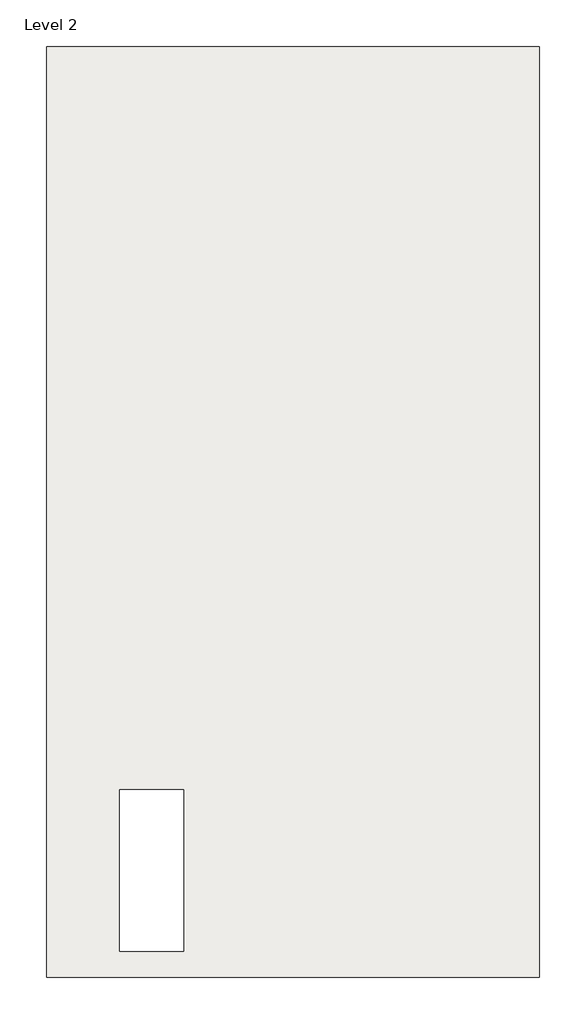
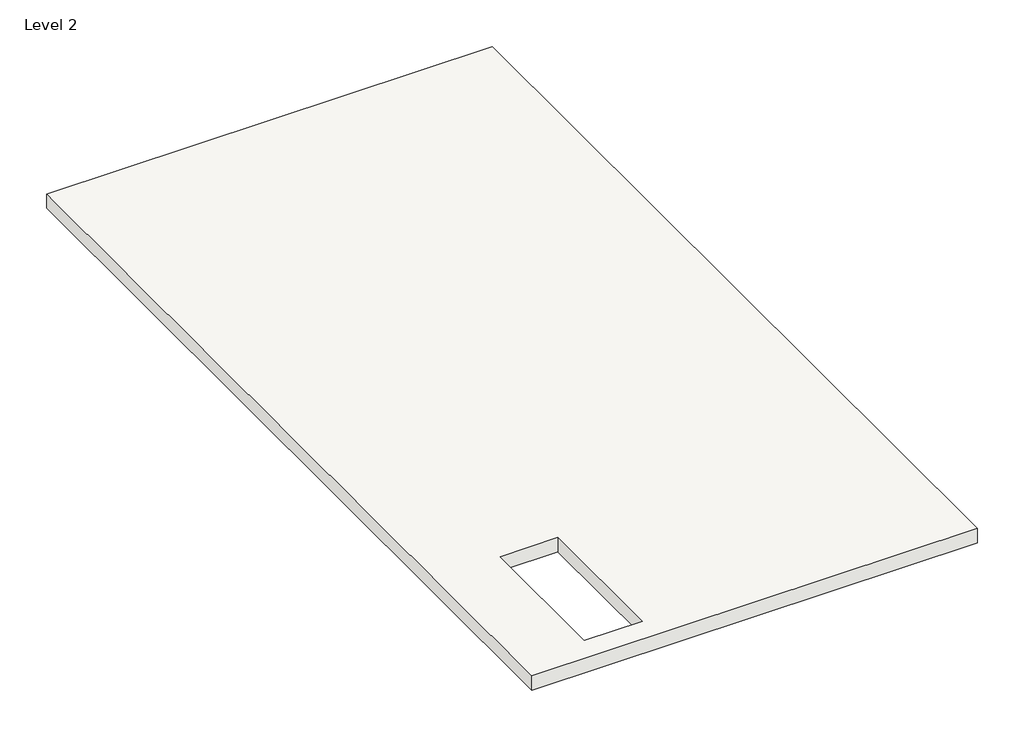
# One storey: 1 roof.
"""IFC4 building model written with IfcOpenShell, lengths in millimetres."""

from ifc_helpers import new_model, si_unit, frame, origin, place, context, project, spatial, polyline, outline, extrude, element, save

model = new_model("IFC4")

# Units and contexts
model_context = context("Model", 3, world=origin())
ifc_project = project(units=[si_unit("LENGTHUNIT", "METRE", prefix="MILLI")], contexts=[model_context])

# Site, building, storey
site = spatial("IfcSite", under=ifc_project)
building = spatial("IfcBuilding", under=site)
storey = spatial("IfcBuildingStorey", under=building, Name="Level 2", Elevation=3048.0)

# Roof
placement = place(None, origin())
element("IfcRoof", 1, ObjectType="Generic - 12\"", at=placement, inside=storey, context=model_context, shape_type="SweptSolid", body=[
    extrude(outline(polyline([(-13227.6589543, 12303.047818), (-4236.0589543, 12303.047818), (-4236.0589543, -4664.152182), (-13227.6589543, -4664.152182), (-13227.6589543, 12303.047818)]), holes=[polyline([(-11894.1589543, -1238.8838739), (-11894.1589543, -4185.2838739), (-10725.7589543, -4185.2838739), (-10725.7589543, -1238.8838739), (-11894.1589543, -1238.8838739)])]), frame((0.0, 0.0, 3048.0), z_axis=(0.0, 0.0, 1.0), x_axis=(1.0, 0.0, 0.0)), (0.0, 0.0, 1.0), 304.8),
])

save(model, "model.ifc")

# Revit data of these elements
# Type "Generic - 12\""
#   Assembly Code = "B1020"
#   Layers, outside or top first: 1' - 0" "Brick, Soldier Course" (function 1)
# Element 1 (IfcRoof, "Generic - 12\"")
#   built-in parameter 1001705 = 11 (stored number, unit not read)
#   built-in parameter 1001710 = 33615
#   Phase Created = New Construction
#   Materials on its faces: "Brick, Soldier Course"
# Materials
#   "Brick, Soldier Course": class "Masonry", colour RGB 170 98 104, transparency 0, Description = "Common brick soldier coursed", Cost = 0
